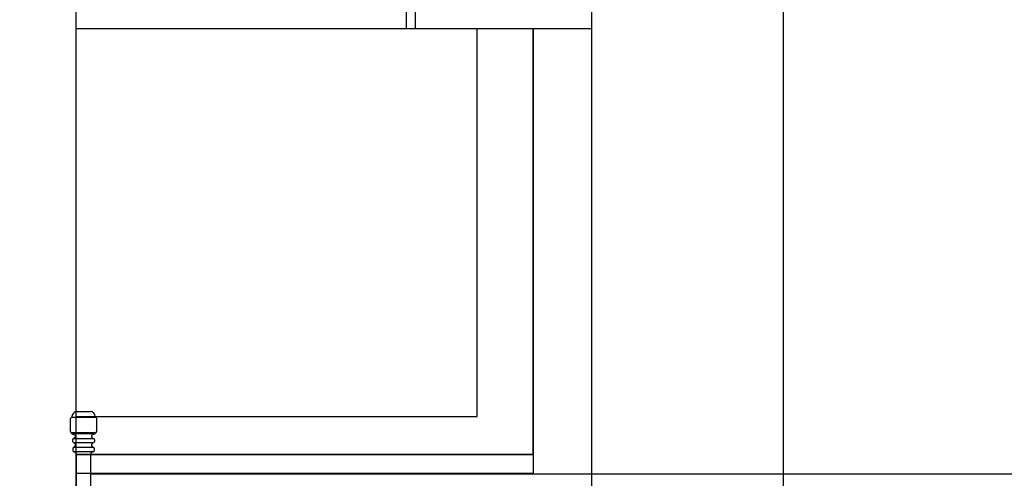
# Model space of a CAD drawing. Units: inches. Extents: x 2278 to 7495, y -71 to 1198.
# Tile 12 of 44: x 4871 to 4938, y 160 to 191. Entities that reach past the tile are written whole.
import ezdxf

# ---------------------------------------------------------------- set-up
doc = ezdxf.new("R2010")
doc.units = ezdxf.units.IN
doc.header["$MEASUREMENT"] = 0
doc.layers.add('A-ANNO-DIMS', color=2, linetype='Continuous', lineweight=18)
doc.layers.add('A-ELEV', color=7, linetype='Continuous', lineweight=25)
doc.styles.get("Standard").update_dxf_attribs({"font": 'arial.ttf'})
doc.dimstyles.get("Standard").update_dxf_attribs({"dimtxt": 6, "dimasz": 3, "dimexe": 0.18, "dimexo": 0.0625, "dimgap": 0.09, "dimtad": 0, "dimtih": 1, "dimtoh": 1, "dimdec": 0, "dimzin": 0, "dimdsep": 46, "dimlunit": 3, "dimtxsty": 'Standard', "dimblk": 'ARCHTICK', "dimcen": 0.09, "dimadec": 0, "dimazin": 0, "dimtfac": 1, "dimtdec": 0, "dimtofl": 0, "dimtmove": 0, "dimatfit": 3, "dimfxl": 1, "dimtolj": 1, "dimtzin": 0, "dimarcsym": 0})

# ---------------------------------------------------------------- blocks, each defined once
blk = doc.blocks.new('_ArchTick')
at = {"color": 0, "linetype": 'ByBlock', "const_width": 0.15}
blk.add_lwpolyline([(-0.5, -0.5), (0.5, 0.5)], dxfattribs=at)
blk = doc.blocks.new('*D123')
at = {"layer": 'A-ANNO-DIMS', "color": 0, "lineweight": -2, "transparency": 16777216}
for p, q in [((4736.95, 340.157), (4736.95, -23.427)), ((5145.676, -1.81), (5145.676, -23.427)), ((4736.95, -23.247), (4923.929, -23.247)), ((5145.676, -23.247), (4958.697, -23.247))]:
    blk.add_line(p, q, dxfattribs=at)
at = {"layer": 'Defpoints', "color": 0, "transparency": 16777216}
for p in [(4736.95, 340.219), (5145.676, -1.747), (5145.676, -23.247)]:
    blk.add_point(p, dxfattribs=at)
at = {"layer": 'A-ANNO-DIMS', "color": 0, "lineweight": -2, "transparency": 16777216, "xscale": 3, "yscale": 3, "zscale": 3, "rotation": 180}
blk.add_blockref('_ArchTick', (4736.95, -23.247), dxfattribs=at)
at = {"layer": 'A-ANNO-DIMS', "color": 0, "lineweight": -2, "transparency": 16777216, "xscale": 3, "yscale": 3, "zscale": 3}
blk.add_blockref('_ArchTick', (5145.676, -23.247), dxfattribs=at)
at = {"layer": 'A-ANNO-DIMS', "color": 0, "transparency": 16777216, "insert": (4941.313, -23.247), "char_height": 6, "attachment_point": 5}
blk.add_mtext('\\A1;34\'-0 1/2"', dxfattribs=at)
blk = doc.blocks.new('*D126')
at = {"layer": 'A-ANNO-DIMS', "color": 0, "lineweight": -2, "transparency": 16777216}
for p, q in [((4837.736, 313.27), (4837.736, 361.899)), ((4837.736, 361.719), (4848.143, 361.719)), ((4874.676, 361.719), (4864.269, 361.719)), ((4874.676, 99.315), (4874.676, 361.899))]:
    blk.add_line(p, q, dxfattribs=at)
at = {"layer": 'Defpoints', "color": 0, "transparency": 16777216}
for p in [(4874.676, 361.719), (4837.736, 313.208), (4874.676, 99.253)]:
    blk.add_point(p, dxfattribs=at)
at = {"layer": 'A-ANNO-DIMS', "color": 0, "lineweight": -2, "transparency": 16777216, "xscale": 3, "yscale": 3, "zscale": 3, "rotation": 180}
blk.add_blockref('_ArchTick', (4837.736, 361.719), dxfattribs=at)
at = {"layer": 'A-ANNO-DIMS', "color": 0, "lineweight": -2, "transparency": 16777216, "xscale": 3, "yscale": 3, "zscale": 3}
blk.add_blockref('_ArchTick', (4874.676, 361.719), dxfattribs=at)
at = {"layer": 'A-ANNO-DIMS', "color": 0, "transparency": 16777216, "insert": (4856.206, 361.719), "char_height": 6, "attachment_point": 5}
blk.add_mtext('\\A1;3\'-1"', dxfattribs=at)
blk = doc.blocks.new('*D127')
at = {"layer": 'A-ANNO-DIMS', "color": 0, "lineweight": -2, "transparency": 16777216}
for p, q in [((4874.676, 99.315), (4874.676, 361.899)), ((4874.676, 361.719), (4881.729, 361.719)), ((4909.676, 361.719), (4902.623, 361.719)), ((4909.676, 99.315), (4909.676, 361.899))]:
    blk.add_line(p, q, dxfattribs=at)
at = {"layer": 'Defpoints', "color": 0, "transparency": 16777216}
for p in [(4909.676, 361.719), (4874.676, 99.253), (4909.676, 99.253)]:
    blk.add_point(p, dxfattribs=at)
at = {"layer": 'A-ANNO-DIMS', "color": 0, "lineweight": -2, "transparency": 16777216, "xscale": 3, "yscale": 3, "zscale": 3, "rotation": 180}
blk.add_blockref('_ArchTick', (4874.676, 361.719), dxfattribs=at)
at = {"layer": 'A-ANNO-DIMS', "color": 0, "lineweight": -2, "transparency": 16777216, "xscale": 3, "yscale": 3, "zscale": 3}
blk.add_blockref('_ArchTick', (4909.676, 361.719), dxfattribs=at)
at = {"layer": 'A-ANNO-DIMS', "color": 0, "transparency": 16777216, "insert": (4892.176, 361.719), "char_height": 6, "attachment_point": 5}
blk.add_mtext('\\A1;2\'-11"', dxfattribs=at)
blk = doc.blocks.new('*D128')
at = {"layer": 'A-ANNO-DIMS', "color": 0, "lineweight": -2, "transparency": 16777216}
for p, q in [((4909.676, 99.315), (4909.676, 361.899)), ((4909.676, 361.719), (4932.111, 361.719)), ((4970.676, 361.719), (4948.241, 361.719)), ((4970.676, 60.779), (4970.676, 361.899))]:
    blk.add_line(p, q, dxfattribs=at)
at = {"layer": 'Defpoints', "color": 0, "transparency": 16777216}
for p in [(4970.676, 361.719), (4909.676, 99.253), (4970.676, 60.717)]:
    blk.add_point(p, dxfattribs=at)
at = {"layer": 'A-ANNO-DIMS', "color": 0, "lineweight": -2, "transparency": 16777216, "xscale": 3, "yscale": 3, "zscale": 3, "rotation": 180}
blk.add_blockref('_ArchTick', (4909.676, 361.719), dxfattribs=at)
at = {"layer": 'A-ANNO-DIMS', "color": 0, "lineweight": -2, "transparency": 16777216, "xscale": 3, "yscale": 3, "zscale": 3}
blk.add_blockref('_ArchTick', (4970.676, 361.719), dxfattribs=at)
at = {"layer": 'A-ANNO-DIMS', "color": 0, "transparency": 16777216, "insert": (4940.176, 361.719), "char_height": 6, "attachment_point": 5}
blk.add_mtext('\\A1;5\'-1"', dxfattribs=at)

msp = doc.modelspace()

# ---------------------------------------------------------------- linework, layer by layer
at = {"layer": 'A-ELEV'}
for p, q in [((4874.676, 124.253), (4874.676, 250.253)), ((4922.676, 66.655), (4922.676, 244.253)), ((4897.076, 225.253), (4897.076, 190.453)), ((4897.676, 225.253), (4897.676, 190.453)), ((4909.676, 190.453), (4909.676, 225.253)), ((4874.676, 190.453), (4909.676, 190.453)), ((4901.887, 164.11), (4901.887, 190.453)), ((4901.887, 164.11), (4901.887, 190.453)), ((4905.676, 190.453), (4905.676, 161.539)), ((4905.676, 190.453), (4905.676, 161.539)), ((4905.676, 190.453), (4905.676, 160.253)), ((4905.676, 190.453), (4905.676, 160.253)), ((4905.676, 190.453), (4905.676, 160.253)), ((4905.676, 161.539), (4905.676, 190.453)), ((4874.724, 164.449), (4875.646, 164.449)), ((4874.298, 163.092), (4874.298, 163.965)), ((4875.989, 164.046), (4874.38, 164.046)), ((4874.394, 164.122), (4874.394, 164.046)), ((4874.676, 164.11), (4901.887, 164.11)), ((4874.676, 164.11), (4901.887, 164.11)), ((4875.975, 164.122), (4875.975, 164.046)), ((4876.071, 163.092), (4876.071, 163.965)), ((4875.989, 163.01), (4874.38, 163.01)), ((4874.394, 162.934), (4874.394, 163.01)), ((4875.975, 162.934), (4875.975, 163.01)), ((4874.394, 162.934), (4874.619, 162.837)), ((4875.975, 162.934), (4874.394, 162.934)), ((4874.533, 162.615), (4874.619, 162.711)), ((4874.533, 162.334), (4874.619, 162.238)), ((4875.975, 162.934), (4875.75, 162.837)), ((4875.836, 162.615), (4875.75, 162.711)), ((4875.836, 162.334), (4875.75, 162.238)), ((4874.533, 162.015), (4874.619, 162.112)), ((4874.533, 161.735), (4874.666, 161.64)), ((4875.836, 161.735), (4875.703, 161.64)), ((4875.836, 162.015), (4875.75, 162.112)), ((4874.676, 161.539), (4905.676, 161.539)), ((4874.676, 161.539), (4905.676, 161.539)), ((4905.676, 161.539), (4874.676, 161.539)), ((4874.696, 147.642), (4874.696, 161.577)), ((4875.673, 147.642), (4875.673, 161.577)), ((4905.676, 160.253), (4874.676, 160.253)), ((4905.676, 160.253), (4874.676, 160.253)), ((4905.676, 160.253), (4874.676, 160.253)), ((4969.039, 160.198), (4875.673, 160.198))]:
    msp.add_line(p, q, dxfattribs=at)
for points in [[(4874.533, 162.615), (4875.836, 162.615, -0.414214), (4875.918, 162.533), (4875.918, 162.416, -0.414214), (4875.836, 162.334), (4874.533, 162.334, -0.414214), (4874.451, 162.416), (4874.451, 162.533, -0.414214)], [(4874.533, 161.735), (4875.836, 161.735, 0.414214), (4875.918, 161.816), (4875.918, 161.934, 0.414214), (4875.836, 162.015), (4874.533, 162.015, 0.414214), (4874.451, 161.934), (4874.451, 161.816, 0.414214)]]:
    msp.add_lwpolyline(points, format="xyb", close=True, dxfattribs=at)
for centre, radius, start, end in [((4874.746, 164.097), 0.352, 93.62058, 175.89193), ((4875.623, 164.097), 0.352, 4.10807, 86.37942), ((4874.38, 163.965), 0.0815, 90, 180), ((4875.989, 163.965), 0.0815, 0, 90), ((4874.38, 163.092), 0.0815, 180, 270), ((4875.989, 163.092), 0.0815, 270, 0), ((4874.567, 162.774), 0.0815, 309.328, 50.672), ((4875.802, 162.774), 0.0815, 129.328, 230.672), ((4874.567, 162.175), 0.0815, 309.328, 50.672), ((4875.802, 162.175), 0.0815, 129.328, 230.672), ((4874.614, 161.577), 0.0815, 0, 50.672), ((4875.755, 161.577), 0.0815, 129.328, 180)]:
    msp.add_arc(centre, radius, start, end, dxfattribs=at)

# ---------------------------------------------------------------- dimensions: what is measured, and where the dimension line sits
at = {"layer": 'A-ANNO-DIMS'}
for base, p1, p2, picture, middle in [((4874.676, 361.719), (4837.736, 313.208), (4874.676, 99.253), '*D126', (4856.206, 361.719)), ((4909.676, 361.719), (4874.676, 99.253), (4909.676, 99.253), '*D127', (4892.176, 361.719)), ((4970.676, 361.719), (4909.676, 99.253), (4970.676, 60.717), '*D128', (4940.176, 361.719)), ((5145.676, -23.247), (4736.95, 340.219), (5145.676, -1.747), '*D123', (4941.313, -23.247))]:
    dim = msp.add_linear_dim(base=base, p1=p1, p2=p2, dimstyle='Standard', override={"dimdec": 1, "dimlfac": 1, "dimrnd": 0, "dimzin": 1, "dimdsep": 46, "dimlunit": 4, "dimfrac": 2}, dxfattribs=at)
    dim.commit()
    dim.dimension.update_dxf_attribs({"geometry": picture, "text_midpoint": middle})

doc.saveas('drawing.dxf')
